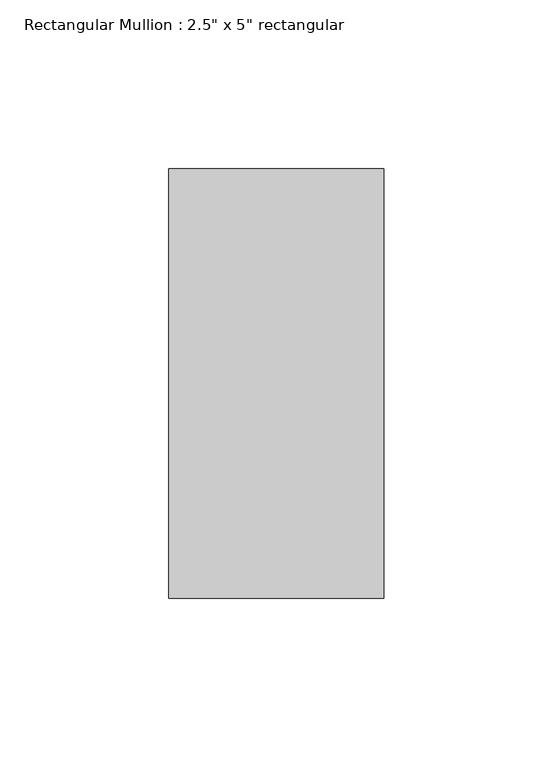
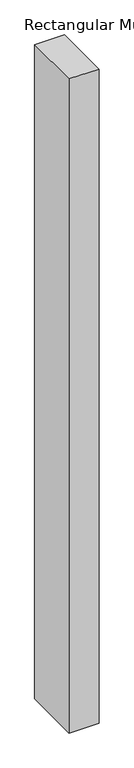
"""IFC4 building model written with IfcOpenShell, lengths in millimetres: member geometry."""

from ifc_helpers import new_model, si_unit, frame, origin, place, context, project, spatial, polyline, outline, extrude, source, transform, mapped, element, save


def member_753b5246(model_context):
    return source(origin(), model_context, "Body", "SweptSolid", [
        extrude(outline(polyline([(0.0, 63.5), (0.0, -63.5), (-63.5, -63.5), (-63.5, 63.5), (0.0, 63.5)])), frame((0.0, 0.0, -1472.6043316), z_axis=(0.0, 0.0, 1.0), x_axis=(1.0, 0.0, 0.0)), (0.0, 0.0, 1.0), 1472.6043316),
    ])


if __name__ == "__main__":
    model = new_model("IFC4")
    model_context = context("Model", 3, world=origin())
    ifc_project = project(units=[si_unit("LENGTHUNIT", "METRE", prefix="MILLI")], contexts=[model_context])
    site = spatial("IfcSite", under=ifc_project)
    building = spatial("IfcBuilding", under=site)
    placement = place(None, origin())
    member_shape = member_753b5246(model_context)
    element("IfcMember", 1, ObjectType="Rectangular Mullion : 2.5\" x 5\" rectangular", at=placement, inside=building, context=model_context, shape_type="MappedRepresentation", body=[
        mapped(member_shape, transform((0.0, 0.0, 0.0), x_axis=(1.0, 0.0, 0.0), y_axis=(0.0, 1.0, 0.0), z_axis=(0.0, 0.0, 1.0))),
    ])
    save(model, "model.ifc")

# Revit data of these elements
# Type "Rectangular Mullion : 2.5\" x 5\" rectangular"
#   built-in parameter 1007304 = 0.416667 (stored number, unit not read)
#   built-in parameter 1007301 = 0.104167 (stored number, unit not read)
#   built-in parameter 1007300 = 0.104167 (stored number, unit not read)
# Element 1 (IfcMember, "Rectangular Mullion : 2.5\" x 5\" rectangular")
#   Materials on its faces: "Aluminum"
# Materials
#   "Aluminum": class "Metal", colour RGB 247 247 247, transparency 0, Description = "Aluminum 6061", Cost = 0
